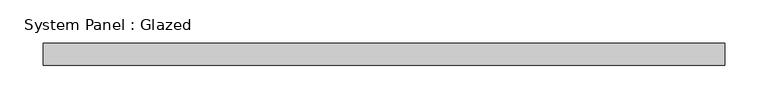
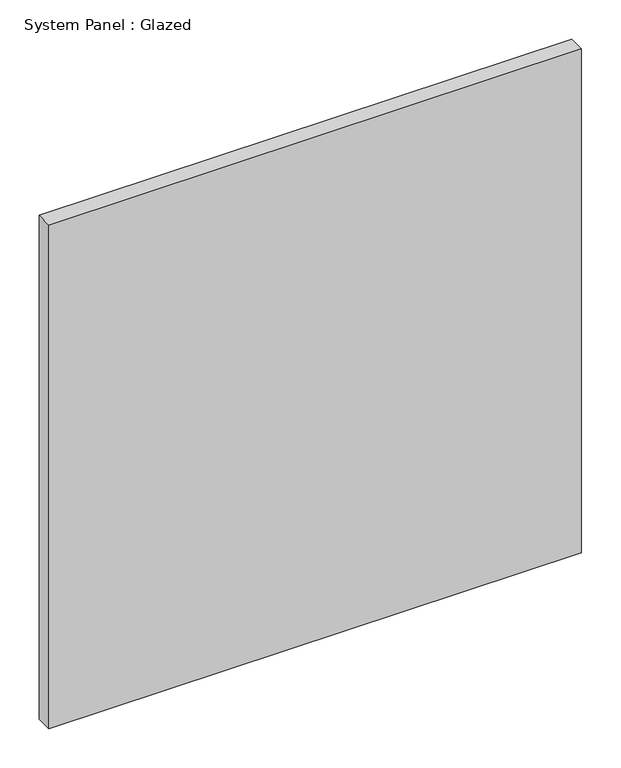
"""IFC4 building model written with IfcOpenShell, lengths in millimetres: plate geometry, System Panel : Glazed."""

from ifc_helpers import new_model, si_unit, origin, origin_with_axes, place, context, project, spatial, polyline, outline, extrude, source, transform, mapped, element, save


def system_panel_glazed_26639370(model_context):
    return source(origin(), model_context, "Body", "SweptSolid", [
        extrude(outline(polyline([(393.7, 19.05), (-393.7, 19.05), (-393.7, 44.45), (393.7, 44.45), (393.7, 19.05)])), origin_with_axes(), (0.0, 0.0, 1.0), 787.4),
    ])


if __name__ == "__main__":
    model = new_model("IFC4")
    model_context = context("Model", 3, world=origin())
    ifc_project = project(units=[si_unit("LENGTHUNIT", "METRE", prefix="MILLI")], contexts=[model_context])
    site = spatial("IfcSite", under=ifc_project)
    building = spatial("IfcBuilding", under=site)
    placement = place(None, origin())
    system_panel_glazed_shape = system_panel_glazed_26639370(model_context)
    element("IfcPlate", 1, ObjectType="System Panel : Glazed", at=placement, inside=building, context=model_context, shape_type="MappedRepresentation", body=[
        mapped(system_panel_glazed_shape, transform((0.0, 0.0, 0.0), x_axis=(1.0, 0.0, 0.0), y_axis=(0.0, 1.0, 0.0), z_axis=(0.0, 0.0, 1.0))),
    ])
    save(model, "model.ifc")

# Revit data of these elements
# Type "System Panel : Glazed"
#   Construction Type Id = "GSP4R"
#   Analytic Construction = "1/8 in Pilkington single glazing"
#   Visual Light Transmittance = 0.9
#   Solar Heat Gain Coefficient = 0.86
#   Heat Transfer Coefficient (U) = 1.18115 BTU/(h·ft²·°F)
#   Define Thermal Properties by = 1
# Element 1 (IfcPlate, "System Panel : Glazed")
#   Materials on its faces: "Glass"
# Materials
#   "Glass": class "Glass", colour RGB 0 128 192, transparency 0.75, Description = "Soda Lime Glass", Cost = 0
